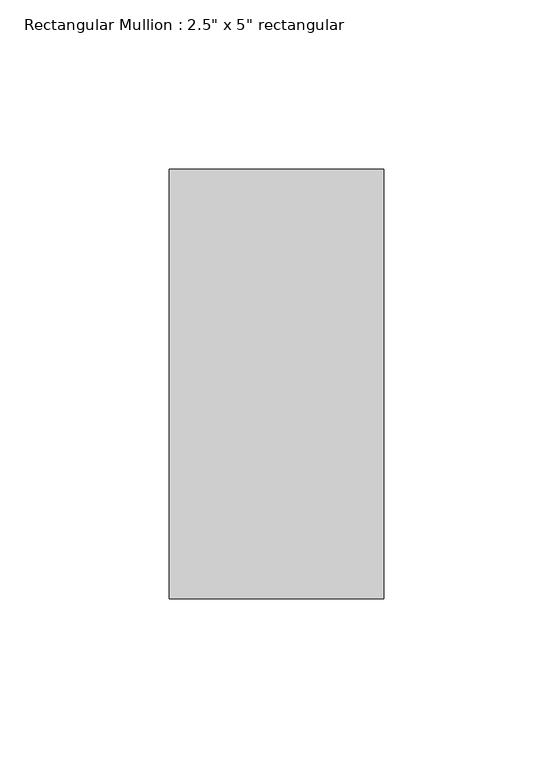
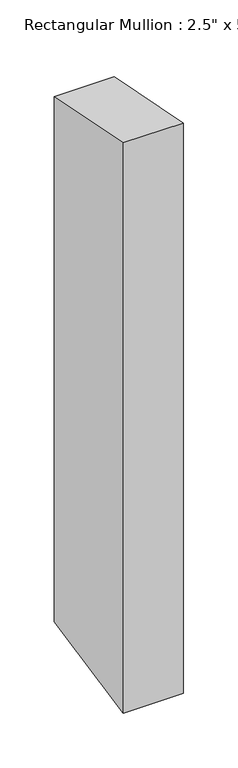
"""IFC4 building model written with IfcOpenShell, lengths in millimetres: member geometry."""

from ifc_helpers import new_model, si_unit, frame, origin, place, context, project, spatial, polyline, outline, extrude, source, transform, mapped, element, save


def member_c6c1cc64(model_context):
    return source(origin(), model_context, "Body", "SweptSolid", [
        extrude(outline(polyline([(-63.5, 12.6309353), (63.5, -12.6309353), (63.5, -602.7536382), (-63.5, -628.0155089), (-63.5, 12.6309353)])), frame((-63.5, 0.0, 0.0), z_axis=(1.0, 0.0, 0.0), x_axis=(0.0, 1.0, 0.0)), (0.0, 0.0, 1.0), 63.5),
    ])


if __name__ == "__main__":
    model = new_model("IFC4")
    model_context = context("Model", 3, world=origin())
    ifc_project = project(units=[si_unit("LENGTHUNIT", "METRE", prefix="MILLI")], contexts=[model_context])
    site = spatial("IfcSite", under=ifc_project)
    building = spatial("IfcBuilding", under=site)
    placement = place(None, origin())
    member_shape = member_c6c1cc64(model_context)
    element("IfcMember", 1, ObjectType="Rectangular Mullion : 2.5\" x 5\" rectangular", at=placement, inside=building, context=model_context, shape_type="MappedRepresentation", body=[
        mapped(member_shape, transform((0.0, 0.0, 0.0), x_axis=(1.0, 0.0, 0.0), y_axis=(0.0, 1.0, 0.0), z_axis=(0.0, 0.0, 1.0))),
    ])
    save(model, "model.ifc")

# Revit data of these elements
# Type "Rectangular Mullion : 2.5\" x 5\" rectangular"
#   built-in parameter 1007304 = 0.416667 (stored number, unit not read)
#   built-in parameter 1007301 = 0.104167 (stored number, unit not read)
#   built-in parameter 1007300 = 0.104167 (stored number, unit not read)
# Element 1 (IfcMember, "Rectangular Mullion : 2.5\" x 5\" rectangular")
#   Materials on its faces: "Iron, Ductile"
# Materials
#   "Iron, Ductile": class "Metal", colour RGB 0 0 0, transparency 0, Description = "Ductile cast iron", Cost = 0
